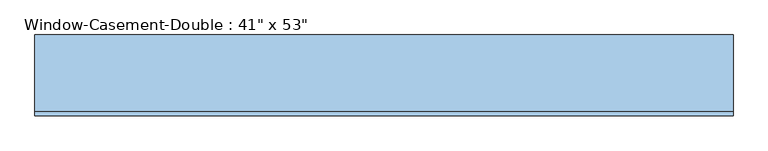
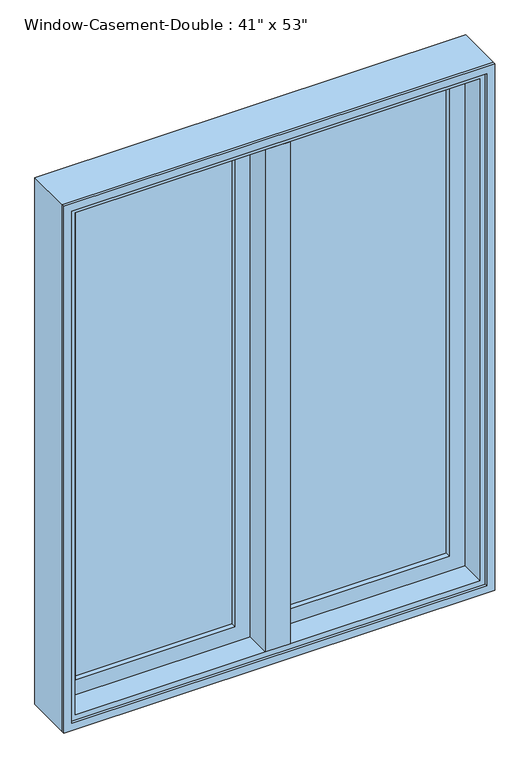
"""IFC4 building model written with IfcOpenShell, lengths in millimetres: window geometry."""

from ifc_helpers import new_model, si_unit, frame, origin, place, context, project, spatial, polyline, outline, extrude, faceted_brep, source, transform, mapped, element, save


def window_6ac8034a(model_context):
    return source(origin(), model_context, "Body", "SolidModel", [
        faceted_brep([(9.525, 69.85, 2247.9), (-9.525, 69.85, 2247.9), (-9.525, 19.05, 2247.9), (9.525, 19.05, 2247.9), (9.525, 69.85, 927.1), (9.525, 19.05, 927.1), (-9.525, 19.05, 927.1), (-9.525, 69.85, 927.1), (-9.525, 19.05, 946.15), (-9.525, 19.05, 2228.85), (-30.1625, 19.05, 946.15), (-30.1625, 19.05, 2228.85), (-30.1625, -44.45, 946.15), (-30.1625, -44.45, 2228.85), (30.1625, -44.45, 946.15), (30.1625, -44.45, 2228.85), (30.1625, 19.05, 946.15), (30.1625, 19.05, 2228.85), (9.525, 19.05, 946.15), (9.525, 19.05, 2228.85)], [[[0, 1, 2, 3]], [[4, 5, 6, 7]], [[1, 0, 4, 7]], [[2, 1, 7, 6, 8, 9]], [[9, 8, 10, 11]], [[11, 10, 12, 13]], [[13, 12, 14, 15]], [[15, 14, 16, 17]], [[17, 16, 18, 19]], [[0, 3, 19, 18, 5, 4]], [[18, 8, 6, 5]], [[9, 19, 3, 2]], [[8, 18, 16, 14, 12, 10]], [[19, 9, 11, 13, 15, 17]]]),
        extrude(outline(polyline([(-66.675, 50.8), (-66.675, 44.45), (-450.85, 44.45), (-450.85, 50.8), (-66.675, 50.8)])), frame((0.0, 0.0, 984.25), z_axis=(0.0, 0.0, 1.0), x_axis=(1.0, 0.0, 0.0)), (0.0, 0.0, 1.0), 1206.5),
        extrude(outline(polyline([(-450.85, 31.75), (-450.85, 38.1), (-66.675, 38.1), (-66.675, 31.75), (-450.85, 31.75)])), frame((0.0, 0.0, 984.25), z_axis=(0.0, 0.0, 1.0), x_axis=(1.0, 0.0, 0.0)), (0.0, 0.0, 1.0), 1206.5),
        extrude(outline(polyline([(450.85, 50.8), (450.85, 44.45), (66.675, 44.45), (66.675, 50.8), (450.85, 50.8)])), frame((0.0, 0.0, 984.25), z_axis=(0.0, 0.0, 1.0), x_axis=(1.0, 0.0, 0.0)), (0.0, 0.0, 1.0), 1206.5),
        extrude(outline(polyline([(66.675, 31.75), (66.675, 38.1), (450.85, 38.1), (450.85, 31.75), (66.675, 31.75)])), frame((0.0, 0.0, 984.25), z_axis=(0.0, 0.0, 1.0), x_axis=(1.0, 0.0, 0.0)), (0.0, 0.0, 1.0), 1206.5),
        extrude(outline(polyline([(2247.9, -508.0), (927.1, -508.0), (927.1, -9.525), (2247.9, -9.525), (2247.9, -508.0)]), holes=[polyline([(2190.75, -66.675), (984.25, -66.675), (984.25, -450.85), (2190.75, -450.85), (2190.75, -66.675)])]), frame((0.0, 19.05, 0.0), z_axis=(0.0, 1.0, 0.0), x_axis=(0.0, 0.0, 1.0)), (0.0, 0.0, 1.0), 44.45),
        extrude(outline(polyline([(927.1, 508.0), (2247.9, 508.0), (2247.9, 9.525), (927.1, 9.525), (927.1, 508.0)]), holes=[polyline([(984.25, 66.675), (2190.75, 66.675), (2190.75, 450.85), (984.25, 450.85), (984.25, 66.675)])]), frame((0.0, 19.05, 0.0), z_axis=(0.0, 1.0, 0.0), x_axis=(0.0, 0.0, 1.0)), (0.0, 0.0, 1.0), 44.45),
        extrude(outline(polyline([(2260.6, -520.7), (914.4, -520.7), (914.4, 520.7), (2260.6, 520.7), (2260.6, -520.7)]), holes=[polyline([(2241.55, 501.65), (933.45, 501.65), (933.45, -501.65), (2241.55, -501.65), (2241.55, 501.65)])]), frame((0.0, -50.8, 0.0), z_axis=(0.0, 1.0, 0.0), x_axis=(0.0, 0.0, 1.0)), (0.0, 0.0, 1.0), 6.35),
        faceted_brep([(488.95, 19.05, 2228.85), (488.95, -44.45, 2228.85), (-488.95, -44.45, 2228.85), (-488.95, 19.05, 2228.85), (508.0, 69.85, 2247.9), (508.0, 19.05, 2247.9), (-508.0, 19.05, 2247.9), (-508.0, 69.85, 2247.9), (520.7, -44.45, 2260.6), (520.7, 69.85, 2260.6), (-520.7, 69.85, 2260.6), (-520.7, -44.45, 2260.6), (-488.95, -44.45, 946.15), (-488.95, 19.05, 946.15), (-508.0, 19.05, 927.1), (-508.0, 69.85, 927.1), (-520.7, 69.85, 914.4), (-520.7, -44.45, 914.4), (488.95, -44.45, 946.15), (488.95, 19.05, 946.15), (508.0, 19.05, 927.1), (508.0, 69.85, 927.1), (520.7, 69.85, 914.4), (520.7, -44.45, 914.4)], [[[0, 1, 2, 3]], [[4, 5, 6, 7]], [[8, 9, 10, 11]], [[3, 2, 12, 13]], [[7, 6, 14, 15]], [[11, 10, 16, 17]], [[13, 12, 18, 19]], [[15, 14, 20, 21]], [[17, 16, 22, 23]], [[11, 17, 23, 8], [1, 18, 12, 2]], [[19, 18, 1, 0]], [[5, 20, 14, 6], [3, 13, 19, 0]], [[21, 20, 5, 4]], [[23, 22, 9, 8]], [[9, 22, 16, 10], [7, 15, 21, 4]]]),
    ])


if __name__ == "__main__":
    model = new_model("IFC4")
    model_context = context("Model", 3, world=origin())
    ifc_project = project(units=[si_unit("LENGTHUNIT", "METRE", prefix="MILLI")], contexts=[model_context])
    site = spatial("IfcSite", under=ifc_project)
    building = spatial("IfcBuilding", under=site)
    placement = place(None, origin())
    window_shape = window_6ac8034a(model_context)
    element("IfcWindow", 1, ObjectType="Window-Casement-Double : 41\" x 53\"", at=placement, inside=building, context=model_context, shape_type="MappedRepresentation", body=[
        mapped(window_shape, transform((0.0, 0.0, 0.0), x_axis=(1.0, 0.0, 0.0), y_axis=(0.0, 1.0, 0.0), z_axis=(0.0, 0.0, 1.0))),
    ])
    save(model, "model.ifc")

# Revit data of these elements
# Type "Window-Casement-Double : 41\" x 53\""
#   Type Mark = "15"
#   Fire Rating = "0.5h"
#   Assembly Code = "B2020100"
#   Analytic Construction = "Double glazing - domestic"
#   Frame Extension [instance default] = 0' - 0 1/4"
#   Window Inset [instance default] = 0' - 0"
#   Wall Thickness [instance default] = 0' - 6"
#   Interior Wall Closure [instance default] = 0' - 2 1/4"
#   Half Width = 1' - 8 1/2"
#   Visual Light Transmittance = 0.81
#   Thermal Resistance (R) = 1.8146 (h·ft²·°F)/BTU
#   Solar Heat Gain Coefficient = 0.76
#   Rough Width = 3' - 5 1/2"
#   Rough Height = 4' - 5 1/2"
#   Height = 4' - 5"
#   Heat Transfer Coefficient (U) = 0.5511 BTU/(h·ft²·°F)
#   Exterior Wall Closure [instance default] = 0' - 1 1/4"
#   Extension Jamb [instance default] = 0' - 2 1/4"
#   Default Sill Height = 3' - 0"
#   Width = 3' - 5"
#   Define Thermal Properties by = 0
#   Muntin Visibility = yes
#   Interior Trim Visibility [instance default] = yes
#   Exterior Trim Visibility [instance default] = yes
#   Extension Jamb Visibility [instance default] = yes
#   Interior Trim Material = Wood - Stained
#   Muntin Pattern = Muntin Pattern_2x2 : Muntin Pattern_2x2
#   Interior Trim = Trim-Window-Interior-Flat : Picture Frame
#   Interior Frame Material = Wood - Stained
#   Glass Panel Material = Glass
#   Exterior Trim = Trim-Window-Exterior-Flat : with Sill
#   Wall Closure = (empty or 0)
# Element 1 (IfcWindow, "Window-Casement-Double : 41\" x 53\"")
#   Wall Thickness = 0' - 4"
#   Extension Jamb = 0' - 0 1/4"
#   Materials on its faces: "Wood - Stained", "Glass"
# Materials
#   "Wood - Stained": class "Wood", colour RGB 224 178 126, transparency 0, Cost = 0
#   "Glass": class "Glass", colour RGB 0 128 192, transparency 0.75, Description = "Soda Lime Glass", Cost = 0
